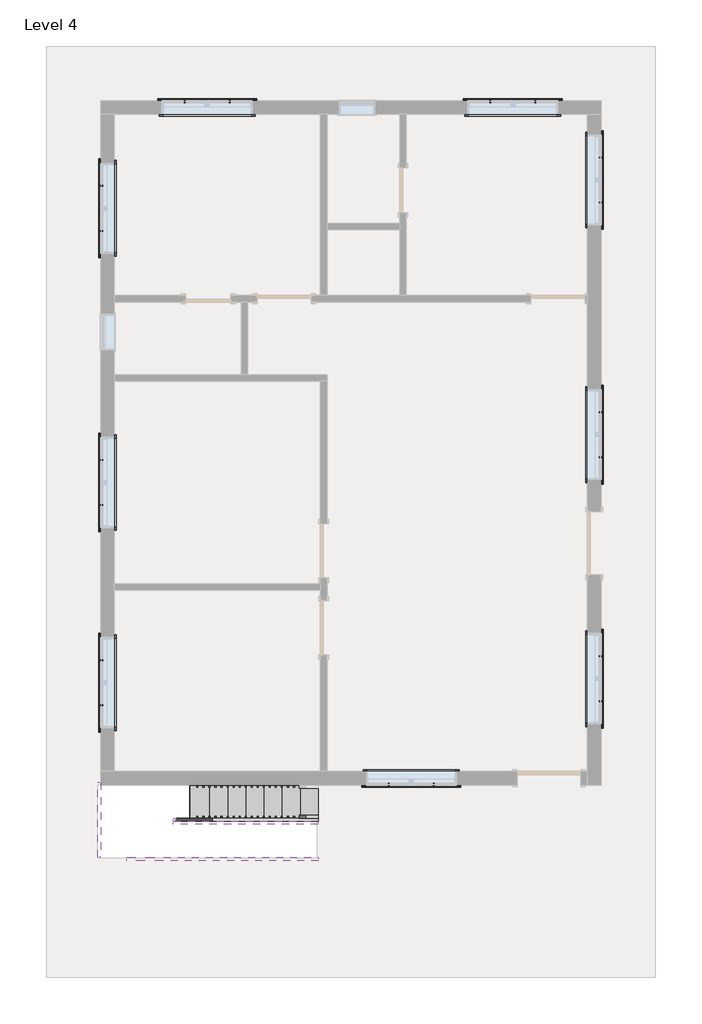
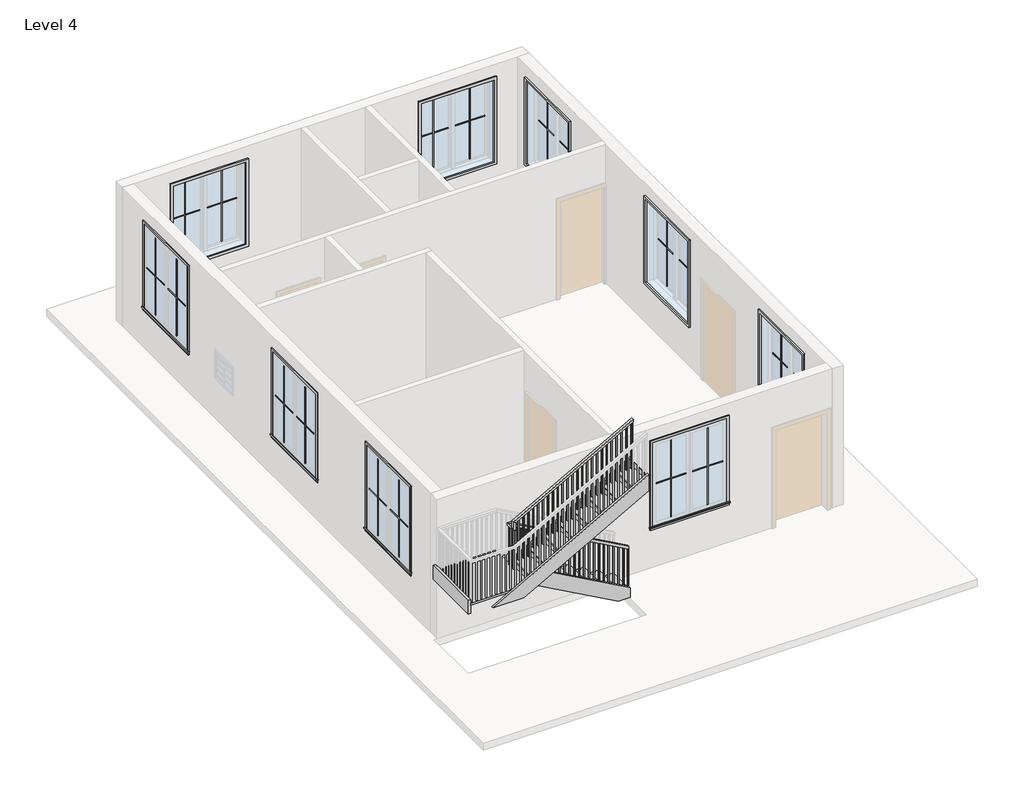
# One storey, part 3 of 3: 36 proxies, 6 members, 1 railing, 1 stair flight.
"""IFC4 building model written with IfcOpenShell, lengths in millimetres."""

from ifc_helpers import new_model, si_unit, frame, origin, place, context, project, spatial, polyline, outline, extrude, faceted_brep, transform, mapped, element, save
from components import muntin_pattern_2x2_muntin_pattern_2x2_f6a80940, muntin_pattern_2x2_muntin_pattern_2x2_09b00a1c, trim_window_exterior_flat_with_sill_698ed857, trim_window_interior_flat_picture_frame_92551a5e, stair_flight_719863f8

model = new_model("IFC4")

# Units and contexts
model_context = context("Model", 3, world=origin())
ifc_project = project(units=[si_unit("LENGTHUNIT", "METRE", prefix="MILLI")], contexts=[model_context])

# Site, building, storey
site = spatial("IfcSite", under=ifc_project)
building = spatial("IfcBuilding", under=site)
storey = spatial("IfcBuildingStorey", under=building, Name="Level 4", Elevation=6400.8)

# Proxies
placement = place(None, origin())
muntin_pattern_2x2_muntin_pattern_2x2_shape = muntin_pattern_2x2_muntin_pattern_2x2_f6a80940(model_context)
element("IfcBuildingElementProxy", 1, Name="Muntin Pattern_2x2 : Muntin Pattern_2x2", ObjectType="Muntin Pattern_2x2 : Muntin Pattern_2x2", at=placement, inside=storey, context=model_context, shape_type="MappedRepresentation", body=[
    mapped(muntin_pattern_2x2_muntin_pattern_2x2_shape, transform((-5453.9948569, -3961.7808037, 7385.05), x_axis=(0.0, 1.0, 0.0), y_axis=(-1.0, 0.0, 0.0), z_axis=(0.0, 0.0, 1.0))),
])
element("IfcBuildingElementProxy", 2, Name="Muntin Pattern_2x2 : Muntin Pattern_2x2", ObjectType="Muntin Pattern_2x2 : Muntin Pattern_2x2", at=placement, inside=storey, context=model_context, shape_type="MappedRepresentation", body=[
    mapped(muntin_pattern_2x2_muntin_pattern_2x2_shape, transform((-5453.9948569, -593.1058037, 7385.05), x_axis=(0.0, 1.0, 0.0), y_axis=(-1.0, 0.0, 0.0), z_axis=(0.0, 0.0, 1.0))),
])
element("IfcBuildingElementProxy", 3, Name="Muntin Pattern_2x2 : Muntin Pattern_2x2", ObjectType="Muntin Pattern_2x2 : Muntin Pattern_2x2", at=placement, inside=storey, context=model_context, shape_type="MappedRepresentation", body=[
    mapped(muntin_pattern_2x2_muntin_pattern_2x2_shape, transform((-5453.9948569, 4023.3441963, 7385.05), x_axis=(0.0, 1.0, 0.0), y_axis=(-1.0, 0.0, 0.0), z_axis=(0.0, 0.0, 1.0))),
])
element("IfcBuildingElementProxy", 4, Name="Muntin Pattern_2x2 : Muntin Pattern_2x2", ObjectType="Muntin Pattern_2x2 : Muntin Pattern_2x2", at=placement, inside=storey, context=model_context, shape_type="MappedRepresentation", body=[
    mapped(muntin_pattern_2x2_muntin_pattern_2x2_shape, transform((2947.0551431, 5258.4191963, 7385.05), x_axis=(0.0, -1.0, 0.0), y_axis=(1.0, 0.0, 0.0), z_axis=(0.0, 0.0, 1.0))),
])
element("IfcBuildingElementProxy", 5, Name="Muntin Pattern_2x2 : Muntin Pattern_2x2", ObjectType="Muntin Pattern_2x2 : Muntin Pattern_2x2", at=placement, inside=storey, context=model_context, shape_type="MappedRepresentation", body=[
    mapped(muntin_pattern_2x2_muntin_pattern_2x2_shape, transform((2947.0551431, 972.1691963, 7385.05), x_axis=(0.0, -1.0, 0.0), y_axis=(1.0, 0.0, 0.0), z_axis=(0.0, 0.0, 1.0))),
])
element("IfcBuildingElementProxy", 6, Name="Muntin Pattern_2x2 : Muntin Pattern_2x2", ObjectType="Muntin Pattern_2x2 : Muntin Pattern_2x2", at=placement, inside=storey, context=model_context, shape_type="MappedRepresentation", body=[
    mapped(muntin_pattern_2x2_muntin_pattern_2x2_shape, transform((2947.0551431, -3136.2808037, 7385.05), x_axis=(0.0, -1.0, 0.0), y_axis=(1.0, 0.0, 0.0), z_axis=(0.0, 0.0, 1.0))),
])
element("IfcBuildingElementProxy", 7, Name="Muntin Pattern_2x2 : Muntin Pattern_2x2", ObjectType="Muntin Pattern_2x2 : Muntin Pattern_2x2", at=placement, inside=storey, context=model_context, shape_type="MappedRepresentation", body=[
    mapped(muntin_pattern_2x2_muntin_pattern_2x2_shape, transform((141.9426431, -5296.8683037, 7385.05), x_axis=(-1.0, 0.0, 0.0), y_axis=(0.0, -1.0, 0.0), z_axis=(0.0, 0.0, 1.0))),
])
element("IfcBuildingElementProxy", 8, Name="Muntin Pattern_2x2 : Muntin Pattern_2x2", ObjectType="Muntin Pattern_2x2 : Muntin Pattern_2x2", at=placement, inside=storey, context=model_context, shape_type="MappedRepresentation", body=[
    mapped(muntin_pattern_2x2_muntin_pattern_2x2_shape, transform((1091.2676431, 6202.9816963, 7385.05), x_axis=(1.0, 0.0, 0.0), y_axis=(0.0, 1.0, 0.0), z_axis=(0.0, 0.0, 1.0))),
])
element("IfcBuildingElementProxy", 9, Name="Muntin Pattern_2x2 : Muntin Pattern_2x2", ObjectType="Muntin Pattern_2x2 : Muntin Pattern_2x2", at=placement, inside=storey, context=model_context, shape_type="MappedRepresentation", body=[
    mapped(muntin_pattern_2x2_muntin_pattern_2x2_shape, transform((-4052.2323569, 6202.9816963, 7385.05), x_axis=(1.0, 0.0, 0.0), y_axis=(0.0, 1.0, 0.0), z_axis=(0.0, 0.0, 1.0))),
])
muntin_pattern_2x2_muntin_pattern_2x2_2_shape = muntin_pattern_2x2_muntin_pattern_2x2_09b00a1c(model_context)
element("IfcBuildingElementProxy", 10, Name="Muntin Pattern_2x2 : Muntin Pattern_2x2", ObjectType="Muntin Pattern_2x2 : Muntin Pattern_2x2", at=placement, inside=storey, context=model_context, shape_type="MappedRepresentation", body=[
    mapped(muntin_pattern_2x2_muntin_pattern_2x2_2_shape, transform((-5453.9948569, -3202.9558037, 7385.05), x_axis=(0.0, -1.0, 0.0), y_axis=(1.0, 0.0, 0.0), z_axis=(0.0, 0.0, 1.0))),
])
element("IfcBuildingElementProxy", 11, Name="Muntin Pattern_2x2 : Muntin Pattern_2x2", ObjectType="Muntin Pattern_2x2 : Muntin Pattern_2x2", at=placement, inside=storey, context=model_context, shape_type="MappedRepresentation", body=[
    mapped(muntin_pattern_2x2_muntin_pattern_2x2_2_shape, transform((-5453.9948569, 165.7191963, 7385.05), x_axis=(0.0, -1.0, 0.0), y_axis=(1.0, 0.0, 0.0), z_axis=(0.0, 0.0, 1.0))),
])
element("IfcBuildingElementProxy", 12, Name="Muntin Pattern_2x2 : Muntin Pattern_2x2", ObjectType="Muntin Pattern_2x2 : Muntin Pattern_2x2", at=placement, inside=storey, context=model_context, shape_type="MappedRepresentation", body=[
    mapped(muntin_pattern_2x2_muntin_pattern_2x2_2_shape, transform((-5453.9948569, 4782.1691963, 7385.05), x_axis=(0.0, -1.0, 0.0), y_axis=(1.0, 0.0, 0.0), z_axis=(0.0, 0.0, 1.0))),
])
element("IfcBuildingElementProxy", 13, Name="Muntin Pattern_2x2 : Muntin Pattern_2x2", ObjectType="Muntin Pattern_2x2 : Muntin Pattern_2x2", at=placement, inside=storey, context=model_context, shape_type="MappedRepresentation", body=[
    mapped(muntin_pattern_2x2_muntin_pattern_2x2_2_shape, transform((2947.0551431, 4499.5941963, 7385.05), x_axis=(0.0, 1.0, 0.0), y_axis=(-1.0, 0.0, 0.0), z_axis=(0.0, 0.0, 1.0))),
])
element("IfcBuildingElementProxy", 14, Name="Muntin Pattern_2x2 : Muntin Pattern_2x2", ObjectType="Muntin Pattern_2x2 : Muntin Pattern_2x2", at=placement, inside=storey, context=model_context, shape_type="MappedRepresentation", body=[
    mapped(muntin_pattern_2x2_muntin_pattern_2x2_2_shape, transform((2947.0551431, 213.3441963, 7385.05), x_axis=(0.0, 1.0, 0.0), y_axis=(-1.0, 0.0, 0.0), z_axis=(0.0, 0.0, 1.0))),
])
element("IfcBuildingElementProxy", 15, Name="Muntin Pattern_2x2 : Muntin Pattern_2x2", ObjectType="Muntin Pattern_2x2 : Muntin Pattern_2x2", at=placement, inside=storey, context=model_context, shape_type="MappedRepresentation", body=[
    mapped(muntin_pattern_2x2_muntin_pattern_2x2_2_shape, transform((2947.0551431, -3895.1058037, 7385.05), x_axis=(0.0, 1.0, 0.0), y_axis=(-1.0, 0.0, 0.0), z_axis=(0.0, 0.0, 1.0))),
])
element("IfcBuildingElementProxy", 16, Name="Muntin Pattern_2x2 : Muntin Pattern_2x2", ObjectType="Muntin Pattern_2x2 : Muntin Pattern_2x2", at=placement, inside=storey, context=model_context, shape_type="MappedRepresentation", body=[
    mapped(muntin_pattern_2x2_muntin_pattern_2x2_2_shape, transform((-616.8823569, -5296.8683037, 7385.05), x_axis=(1.0, 0.0, 0.0), y_axis=(0.0, 1.0, 0.0), z_axis=(0.0, 0.0, 1.0))),
])
element("IfcBuildingElementProxy", 17, Name="Muntin Pattern_2x2 : Muntin Pattern_2x2", ObjectType="Muntin Pattern_2x2 : Muntin Pattern_2x2", at=placement, inside=storey, context=model_context, shape_type="MappedRepresentation", body=[
    mapped(muntin_pattern_2x2_muntin_pattern_2x2_2_shape, transform((1850.0926431, 6202.9816963, 7385.05), x_axis=(-1.0, 0.0, 0.0), y_axis=(0.0, -1.0, 0.0), z_axis=(0.0, 0.0, 1.0))),
])
element("IfcBuildingElementProxy", 18, Name="Muntin Pattern_2x2 : Muntin Pattern_2x2", ObjectType="Muntin Pattern_2x2 : Muntin Pattern_2x2", at=placement, inside=storey, context=model_context, shape_type="MappedRepresentation", body=[
    mapped(muntin_pattern_2x2_muntin_pattern_2x2_2_shape, transform((-3293.4073569, 6202.9816963, 7385.05), x_axis=(-1.0, 0.0, 0.0), y_axis=(0.0, -1.0, 0.0), z_axis=(0.0, 0.0, 1.0))),
])
trim_window_exterior_flat_with_sill_shape = trim_window_exterior_flat_with_sill_698ed857(model_context)
element("IfcBuildingElementProxy", 19, Name="Trim-Window-Exterior-Flat : with Sill", ObjectType="Trim-Window-Exterior-Flat : with Sill", at=placement, inside=storey, context=model_context, shape_type="MappedRepresentation", body=[
    mapped(trim_window_exterior_flat_with_sill_shape, transform((-5463.5198569, -3582.3683037, 9144.0), x_axis=(0.0, -1.0, 0.0), y_axis=(0.0, 0.0, 1.0), z_axis=(-1.0, 0.0, 0.0))),
])
element("IfcBuildingElementProxy", 20, Name="Trim-Window-Exterior-Flat : with Sill", ObjectType="Trim-Window-Exterior-Flat : with Sill", at=placement, inside=storey, context=model_context, shape_type="MappedRepresentation", body=[
    mapped(trim_window_exterior_flat_with_sill_shape, transform((-5463.5198569, -213.6933037, 9144.0), x_axis=(0.0, -1.0, 0.0), y_axis=(0.0, 0.0, 1.0), z_axis=(-1.0, 0.0, 0.0))),
])
element("IfcBuildingElementProxy", 21, Name="Trim-Window-Exterior-Flat : with Sill", ObjectType="Trim-Window-Exterior-Flat : with Sill", at=placement, inside=storey, context=model_context, shape_type="MappedRepresentation", body=[
    mapped(trim_window_exterior_flat_with_sill_shape, transform((-5463.5198569, 4402.7566963, 9144.0), x_axis=(0.0, -1.0, 0.0), y_axis=(0.0, 0.0, 1.0), z_axis=(-1.0, 0.0, 0.0))),
])
element("IfcBuildingElementProxy", 22, Name="Trim-Window-Exterior-Flat : with Sill", ObjectType="Trim-Window-Exterior-Flat : with Sill", at=placement, inside=storey, context=model_context, shape_type="MappedRepresentation", body=[
    mapped(trim_window_exterior_flat_with_sill_shape, transform((2956.5801431, 4879.0066963, 9144.0), x_axis=(0.0, 1.0, 0.0), y_axis=(0.0, 0.0, 1.0), z_axis=(1.0, 0.0, 0.0))),
])
element("IfcBuildingElementProxy", 23, Name="Trim-Window-Exterior-Flat : with Sill", ObjectType="Trim-Window-Exterior-Flat : with Sill", at=placement, inside=storey, context=model_context, shape_type="MappedRepresentation", body=[
    mapped(trim_window_exterior_flat_with_sill_shape, transform((2956.5801431, 592.7566963, 9144.0), x_axis=(0.0, 1.0, 0.0), y_axis=(0.0, 0.0, 1.0), z_axis=(1.0, 0.0, 0.0))),
])
element("IfcBuildingElementProxy", 24, Name="Trim-Window-Exterior-Flat : with Sill", ObjectType="Trim-Window-Exterior-Flat : with Sill", at=placement, inside=storey, context=model_context, shape_type="MappedRepresentation", body=[
    mapped(trim_window_exterior_flat_with_sill_shape, transform((2956.5801431, -3515.6933037, 9144.0), x_axis=(0.0, 1.0, 0.0), y_axis=(0.0, 0.0, 1.0), z_axis=(1.0, 0.0, 0.0))),
])
element("IfcBuildingElementProxy", 25, Name="Trim-Window-Exterior-Flat : with Sill", ObjectType="Trim-Window-Exterior-Flat : with Sill", at=placement, inside=storey, context=model_context, shape_type="MappedRepresentation", body=[
    mapped(trim_window_exterior_flat_with_sill_shape, transform((-237.4698569, -5306.3933037, 9144.0), x_axis=(1.0, 0.0, 0.0), y_axis=(0.0, 0.0, 1.0), z_axis=(0.0, -1.0, 0.0))),
])
element("IfcBuildingElementProxy", 26, Name="Trim-Window-Exterior-Flat : with Sill", ObjectType="Trim-Window-Exterior-Flat : with Sill", at=placement, inside=storey, context=model_context, shape_type="MappedRepresentation", body=[
    mapped(trim_window_exterior_flat_with_sill_shape, transform((1470.6801431, 6212.5066963, 9144.0), x_axis=(-1.0, 0.0, 0.0), y_axis=(0.0, 0.0, 1.0), z_axis=(0.0, 1.0, 0.0))),
])
element("IfcBuildingElementProxy", 27, Name="Trim-Window-Exterior-Flat : with Sill", ObjectType="Trim-Window-Exterior-Flat : with Sill", at=placement, inside=storey, context=model_context, shape_type="MappedRepresentation", body=[
    mapped(trim_window_exterior_flat_with_sill_shape, transform((-3672.8198569, 6212.5066963, 9144.0), x_axis=(-1.0, 0.0, 0.0), y_axis=(0.0, 0.0, 1.0), z_axis=(0.0, 1.0, 0.0))),
])
trim_window_interior_flat_picture_frame_shape = trim_window_interior_flat_picture_frame_92551a5e(model_context)
element("IfcBuildingElementProxy", 28, Name="Trim-Window-Interior-Flat : Picture Frame", ObjectType="Trim-Window-Interior-Flat : Picture Frame", at=placement, inside=storey, context=model_context, shape_type="MappedRepresentation", body=[
    mapped(trim_window_interior_flat_picture_frame_shape, transform((-5234.9198569, -3582.3683037, 9144.0), x_axis=(0.0, 1.0, 0.0), y_axis=(0.0, 0.0, 1.0), z_axis=(1.0, 0.0, 0.0))),
])
element("IfcBuildingElementProxy", 29, Name="Trim-Window-Interior-Flat : Picture Frame", ObjectType="Trim-Window-Interior-Flat : Picture Frame", at=placement, inside=storey, context=model_context, shape_type="MappedRepresentation", body=[
    mapped(trim_window_interior_flat_picture_frame_shape, transform((-5234.9198569, -213.6933037, 9144.0), x_axis=(0.0, 1.0, 0.0), y_axis=(0.0, 0.0, 1.0), z_axis=(1.0, 0.0, 0.0))),
])
element("IfcBuildingElementProxy", 30, Name="Trim-Window-Interior-Flat : Picture Frame", ObjectType="Trim-Window-Interior-Flat : Picture Frame", at=placement, inside=storey, context=model_context, shape_type="MappedRepresentation", body=[
    mapped(trim_window_interior_flat_picture_frame_shape, transform((-5234.9198569, 4402.7566963, 9144.0), x_axis=(0.0, 1.0, 0.0), y_axis=(0.0, 0.0, 1.0), z_axis=(1.0, 0.0, 0.0))),
])
element("IfcBuildingElementProxy", 31, Name="Trim-Window-Interior-Flat : Picture Frame", ObjectType="Trim-Window-Interior-Flat : Picture Frame", at=placement, inside=storey, context=model_context, shape_type="MappedRepresentation", body=[
    mapped(trim_window_interior_flat_picture_frame_shape, transform((2727.9801431, 4879.0066963, 9144.0), x_axis=(0.0, -1.0, 0.0), y_axis=(0.0, 0.0, 1.0), z_axis=(-1.0, 0.0, 0.0))),
])
element("IfcBuildingElementProxy", 32, Name="Trim-Window-Interior-Flat : Picture Frame", ObjectType="Trim-Window-Interior-Flat : Picture Frame", at=placement, inside=storey, context=model_context, shape_type="MappedRepresentation", body=[
    mapped(trim_window_interior_flat_picture_frame_shape, transform((2727.9801431, 592.7566963, 9144.0), x_axis=(0.0, -1.0, 0.0), y_axis=(0.0, 0.0, 1.0), z_axis=(-1.0, 0.0, 0.0))),
])
element("IfcBuildingElementProxy", 33, Name="Trim-Window-Interior-Flat : Picture Frame", ObjectType="Trim-Window-Interior-Flat : Picture Frame", at=placement, inside=storey, context=model_context, shape_type="MappedRepresentation", body=[
    mapped(trim_window_interior_flat_picture_frame_shape, transform((2727.9801431, -3515.6933037, 9144.0), x_axis=(0.0, -1.0, 0.0), y_axis=(0.0, 0.0, 1.0), z_axis=(-1.0, 0.0, 0.0))),
])
element("IfcBuildingElementProxy", 34, Name="Trim-Window-Interior-Flat : Picture Frame", ObjectType="Trim-Window-Interior-Flat : Picture Frame", at=placement, inside=storey, context=model_context, shape_type="MappedRepresentation", body=[
    mapped(trim_window_interior_flat_picture_frame_shape, transform((-237.4698569, -5077.7933037, 9144.0), x_axis=(-1.0, 0.0, 0.0), y_axis=(0.0, 0.0, 1.0), z_axis=(0.0, 1.0, 0.0))),
])
element("IfcBuildingElementProxy", 35, Name="Trim-Window-Interior-Flat : Picture Frame", ObjectType="Trim-Window-Interior-Flat : Picture Frame", at=placement, inside=storey, context=model_context, shape_type="MappedRepresentation", body=[
    mapped(trim_window_interior_flat_picture_frame_shape, transform((1470.6801431, 5983.9066963, 9144.0), x_axis=(1.0, 0.0, 0.0), y_axis=(0.0, 0.0, 1.0), z_axis=(0.0, -1.0, 0.0))),
])
element("IfcBuildingElementProxy", 36, Name="Trim-Window-Interior-Flat : Picture Frame", ObjectType="Trim-Window-Interior-Flat : Picture Frame", at=placement, inside=storey, context=model_context, shape_type="MappedRepresentation", body=[
    mapped(trim_window_interior_flat_picture_frame_shape, transform((-3672.8198569, 5983.9066963, 9144.0), x_axis=(1.0, 0.0, 0.0), y_axis=(0.0, 0.0, 1.0), z_axis=(0.0, -1.0, 0.0))),
])

# Members
element("IfcMember", 37, ObjectType="Stringer - 2\" Width", at=placement, inside=storey, context=model_context, shape_type="SweptSolid", body=[
    extrude(outline(polyline([(6400.8, -1805.9198569), (6608.3983948, -1805.9198569), (7934.8428392, -4193.5198569), (7586.1641651, -4193.5198569), (6400.8, -2059.8643597), (6400.8, -1805.9198569)])), frame((0.0, -5915.9933037, 0.0), z_axis=(0.0, 1.0, 0.0), x_axis=(0.0, 0.0, 1.0)), (0.0, 0.0, 1.0), 50.8),
])
element("IfcMember", 38, ObjectType="Stringer - 2\" Width", at=placement, inside=storey, context=model_context, shape_type="SweptSolid", body=[
    extrude(outline(polyline([(-4244.3198569, -5865.1933037), (-4193.5198569, -5865.1933037), (-4193.5198569, -5915.9933037), (-4244.3198569, -5915.9933037), (-4244.3198569, -5865.1933037)])), frame((0.0, 0.0, 7696.2), z_axis=(0.0, 0.0, 1.0), x_axis=(1.0, 0.0, 0.0)), (0.0, 0.0, 1.0), 304.8),
])
element("IfcMember", 39, ObjectType="Stringer - 2\" Width", at=placement, inside=storey, context=model_context, shape_type="SweptSolid", body=[
    extrude(outline(polyline([(8132.3983948, -4244.3198569), (7783.7197207, -4244.3198569), (9138.3863873, -1805.9198569), (9487.0650614, -1805.9198569), (8132.3983948, -4244.3198569)])), frame((0.0, -5966.7933037, 0.0), z_axis=(0.0, 1.0, 0.0), x_axis=(0.0, 0.0, 1.0)), (0.0, 0.0, 1.0), 50.8),
])
element("IfcMember", 40, ObjectType="Stringer - 2\" Width", at=placement, inside=storey, context=model_context, shape_type="SweptSolid", body=[
    extrude(outline(polyline([(6400.8, -1805.9198569), (6608.3983948, -1805.9198569), (8001.0, -4312.6027463), (8001.0, -4940.2243597), (6400.8, -2059.8643597), (6400.8, -1805.9198569)])), frame((0.0, -5306.3933037, 0.0), z_axis=(0.0, 1.0, 0.0), x_axis=(0.0, 0.0, 1.0)), (0.0, 0.0, 1.0), 50.8),
])
element("IfcMember", 41, ObjectType="Stringer - 2\" Width", at=placement, inside=storey, context=model_context, shape_type="SweptSolid", body=[
    extrude(outline(polyline([(-5514.3198569, -5255.5933037), (-5463.5198569, -5255.5933037), (-5463.5198569, -6525.5933037), (-5514.3198569, -6525.5933037), (-5514.3198569, -5255.5933037)])), frame((0.0, 0.0, 7696.2), z_axis=(0.0, 0.0, 1.0), x_axis=(1.0, 0.0, 0.0)), (0.0, 0.0, 1.0), 304.8),
])
element("IfcMember", 42, ObjectType="Stringer - 2\" Width", at=placement, inside=storey, context=model_context, shape_type="SweptSolid", body=[
    extrude(outline(polyline([(7696.2, -4401.8553541), (9138.3863873, -1805.9198569), (9487.0650614, -1805.9198569), (7696.2, -5029.4769675), (7696.2, -4401.8553541)])), frame((0.0, -6576.3933037, 0.0), z_axis=(0.0, 1.0, 0.0), x_axis=(0.0, 0.0, 1.0)), (0.0, 0.0, 1.0), 50.8),
])

# Railing
element("IfcRailing", 43, ObjectType="Handrail - Rectangular", at=placement, inside=storey, context=model_context, shape_type="SolidModel", body=[
    faceted_brep([(-1805.9198569, -5865.1933037, 7484.5333333), (-1805.9198569, -5865.1933037, 7426.420221), (-1805.9198569, -5814.3933037, 7426.420221), (-1805.9198569, -5814.3933037, 7484.5333333), (-4168.1198569, -5865.1933037, 8796.8666667), (-4218.9198569, -5865.1933037, 8766.9757765), (-4218.9198569, -5814.3933037, 8766.9757765), (-4168.1198569, -5814.3933037, 8796.8666667), (-4168.1198569, -5865.1933037, 8839.2), (-4218.9198569, -5865.1933037, 8788.4), (-4218.9198569, -5814.3933037, 8788.4), (-4168.1198569, -5814.3933037, 8839.2), (-4244.3198569, -5865.1933037, 8839.2), (-4244.3198569, -5865.1933037, 8788.4), (-4295.1198569, -5814.3933037, 8788.4), (-4295.1198569, -5814.3933037, 8839.2), (-4244.3198569, -5941.3933037, 8839.2), (-4244.3198569, -5941.3933037, 8788.4), (-4295.1198569, -5941.3933037, 8788.4), (-4295.1198569, -5941.3933037, 8839.2), (-4244.3198569, -5966.7933037, 8839.2), (-4295.1198569, -5966.7933037, 8839.2), (-4295.1198569, -6017.5933037, 8788.4), (-4244.3198569, -6017.5933037, 8788.4)], [[[0, 1, 2, 3]], [[1, 0, 4, 5]], [[2, 1, 5, 6]], [[3, 2, 6, 7]], [[0, 3, 7, 4]], [[5, 4, 8, 9]], [[6, 5, 9, 10]], [[7, 6, 10, 11]], [[4, 7, 11, 8]], [[9, 8, 12, 13]], [[10, 9, 13, 14]], [[11, 10, 14, 15]], [[8, 11, 15, 12]], [[13, 12, 16, 17]], [[14, 13, 17, 18]], [[15, 14, 18, 19]], [[12, 15, 19, 16]], [[20, 21, 22, 23]], [[17, 16, 20, 23]], [[18, 17, 23, 22]], [[19, 18, 22, 21]], [[16, 19, 21, 20]]]),
    faceted_brep([(-4244.3198569, -5966.7933037, 8839.2), (-4244.3198569, -6017.5933037, 8788.4), (-4295.1198569, -6017.5933037, 8788.4), (-4295.1198569, -5966.7933037, 8839.2), (-4244.3198569, -5966.7933037, 8950.420221), (-4295.1198569, -5966.7933037, 8980.3111111), (-4295.1198569, -6017.5933037, 8980.3111111), (-4244.3198569, -6017.5933037, 8950.420221)], [[[0, 1, 2, 3]], [[4, 5, 6, 7]], [[1, 0, 4, 7]], [[2, 1, 7, 6]], [[3, 2, 6, 5]], [[0, 3, 5, 4]]]),
    faceted_brep([(-4295.1198569, -5966.7933037, 8980.3111111), (-4244.3198569, -5966.7933037, 8950.420221), (-4244.3198569, -6017.5933037, 8950.420221), (-4295.1198569, -6017.5933037, 8980.3111111), (-1805.9198569, -5966.7933037, 10363.2), (-1805.9198569, -6017.5933037, 10363.2), (-1805.9198569, -6017.5933037, 10305.0868876), (-1805.9198569, -5966.7933037, 10305.0868876)], [[[0, 1, 2, 3]], [[4, 5, 6, 7]], [[1, 0, 4, 7]], [[2, 1, 7, 6]], [[3, 2, 6, 5]], [[0, 3, 5, 4]]]),
    extrude(outline(polyline([(10285.6841099, -1840.8448569), (9279.4666667, -1840.8448569), (9279.4666667, -1821.7948569), (10296.2674432, -1821.7948569), (10285.6841099, -1840.8448569)])), frame((0.0, -6001.7183037, 0.0), z_axis=(0.0, 1.0, 0.0), x_axis=(0.0, 0.0, 1.0)), (0.0, 0.0, 1.0), 19.05),
    extrude(outline(polyline([(10229.2396654, -1942.4448569), (9279.4666667, -1942.4448569), (9279.4666667, -1923.3948569), (10239.8229988, -1923.3948569), (10229.2396654, -1942.4448569)])), frame((0.0, -6001.7183037, 0.0), z_axis=(0.0, 1.0, 0.0), x_axis=(0.0, 0.0, 1.0)), (0.0, 0.0, 1.0), 19.05),
    extrude(outline(polyline([(10172.795221, -2044.0448569), (9279.4666667, -2044.0448569), (9279.4666667, -2024.9948569), (10183.3785543, -2024.9948569), (10172.795221, -2044.0448569)])), frame((0.0, -6001.7183037, 0.0), z_axis=(0.0, 1.0, 0.0), x_axis=(0.0, 0.0, 1.0)), (0.0, 0.0, 1.0), 19.05),
    extrude(outline(polyline([(10116.3507765, -2145.6448569), (9110.1333333, -2145.6448569), (9110.1333333, -2126.5948569), (10126.9341099, -2126.5948569), (10116.3507765, -2145.6448569)])), frame((0.0, -6001.7183037, 0.0), z_axis=(0.0, 1.0, 0.0), x_axis=(0.0, 0.0, 1.0)), (0.0, 0.0, 1.0), 19.05),
    extrude(outline(polyline([(10059.9063321, -2247.2448569), (9110.1333333, -2247.2448569), (9110.1333333, -2228.1948569), (10070.4896654, -2228.1948569), (10059.9063321, -2247.2448569)])), frame((0.0, -6001.7183037, 0.0), z_axis=(0.0, 1.0, 0.0), x_axis=(0.0, 0.0, 1.0)), (0.0, 0.0, 1.0), 19.05),
    extrude(outline(polyline([(10003.4618876, -2348.8448569), (9110.1333333, -2348.8448569), (9110.1333333, -2329.7948569), (10014.045221, -2329.7948569), (10003.4618876, -2348.8448569)])), frame((0.0, -6001.7183037, 0.0), z_axis=(0.0, 1.0, 0.0), x_axis=(0.0, 0.0, 1.0)), (0.0, 0.0, 1.0), 19.05),
    extrude(outline(polyline([(9947.0174432, -2450.4448569), (8940.8, -2450.4448569), (8940.8, -2431.3948569), (9957.6007765, -2431.3948569), (9947.0174432, -2450.4448569)])), frame((0.0, -6001.7183037, 0.0), z_axis=(0.0, 1.0, 0.0), x_axis=(0.0, 0.0, 1.0)), (0.0, 0.0, 1.0), 19.05),
    extrude(outline(polyline([(9890.5729988, -2552.0448569), (8940.8, -2552.0448569), (8940.8, -2532.9948569), (9901.1563321, -2532.9948569), (9890.5729988, -2552.0448569)])), frame((0.0, -6001.7183037, 0.0), z_axis=(0.0, 1.0, 0.0), x_axis=(0.0, 0.0, 1.0)), (0.0, 0.0, 1.0), 19.05),
    extrude(outline(polyline([(9834.1285543, -2653.6448569), (8940.8, -2653.6448569), (8940.8, -2634.5948569), (9844.7118876, -2634.5948569), (9834.1285543, -2653.6448569)])), frame((0.0, -6001.7183037, 0.0), z_axis=(0.0, 1.0, 0.0), x_axis=(0.0, 0.0, 1.0)), (0.0, 0.0, 1.0), 19.05),
    extrude(outline(polyline([(9777.6841099, -2755.2448569), (8771.4666667, -2755.2448569), (8771.4666667, -2736.1948569), (9788.2674432, -2736.1948569), (9777.6841099, -2755.2448569)])), frame((0.0, -6001.7183037, 0.0), z_axis=(0.0, 1.0, 0.0), x_axis=(0.0, 0.0, 1.0)), (0.0, 0.0, 1.0), 19.05),
    extrude(outline(polyline([(9721.2396654, -2856.8448569), (8771.4666667, -2856.8448569), (8771.4666667, -2837.7948569), (9731.8229988, -2837.7948569), (9721.2396654, -2856.8448569)])), frame((0.0, -6001.7183037, 0.0), z_axis=(0.0, 1.0, 0.0), x_axis=(0.0, 0.0, 1.0)), (0.0, 0.0, 1.0), 19.05),
    extrude(outline(polyline([(9664.795221, -2958.4448569), (8771.4666667, -2958.4448569), (8771.4666667, -2939.3948569), (9675.3785543, -2939.3948569), (9664.795221, -2958.4448569)])), frame((0.0, -6001.7183037, 0.0), z_axis=(0.0, 1.0, 0.0), x_axis=(0.0, 0.0, 1.0)), (0.0, 0.0, 1.0), 19.05),
    extrude(outline(polyline([(9608.3507765, -3060.0448569), (8602.1333333, -3060.0448569), (8602.1333333, -3040.9948569), (9618.9341099, -3040.9948569), (9608.3507765, -3060.0448569)])), frame((0.0, -6001.7183037, 0.0), z_axis=(0.0, 1.0, 0.0), x_axis=(0.0, 0.0, 1.0)), (0.0, 0.0, 1.0), 19.05),
    extrude(outline(polyline([(9551.9063321, -3161.6448569), (8602.1333333, -3161.6448569), (8602.1333333, -3142.5948569), (9562.4896654, -3142.5948569), (9551.9063321, -3161.6448569)])), frame((0.0, -6001.7183037, 0.0), z_axis=(0.0, 1.0, 0.0), x_axis=(0.0, 0.0, 1.0)), (0.0, 0.0, 1.0), 19.05),
    extrude(outline(polyline([(9495.4618876, -3263.2448569), (8602.1333333, -3263.2448569), (8602.1333333, -3244.1948569), (9506.045221, -3244.1948569), (9495.4618876, -3263.2448569)])), frame((0.0, -6001.7183037, 0.0), z_axis=(0.0, 1.0, 0.0), x_axis=(0.0, 0.0, 1.0)), (0.0, 0.0, 1.0), 19.05),
    extrude(outline(polyline([(9439.0174432, -3364.8448569), (8432.8, -3364.8448569), (8432.8, -3345.7948569), (9449.6007765, -3345.7948569), (9439.0174432, -3364.8448569)])), frame((0.0, -6001.7183037, 0.0), z_axis=(0.0, 1.0, 0.0), x_axis=(0.0, 0.0, 1.0)), (0.0, 0.0, 1.0), 19.05),
    extrude(outline(polyline([(9382.5729988, -3466.4448569), (8432.8, -3466.4448569), (8432.8, -3447.3948569), (9393.1563321, -3447.3948569), (9382.5729988, -3466.4448569)])), frame((0.0, -6001.7183037, 0.0), z_axis=(0.0, 1.0, 0.0), x_axis=(0.0, 0.0, 1.0)), (0.0, 0.0, 1.0), 19.05),
    extrude(outline(polyline([(9326.1285543, -3568.0448569), (8432.8, -3568.0448569), (8432.8, -3548.9948569), (9336.7118876, -3548.9948569), (9326.1285543, -3568.0448569)])), frame((0.0, -6001.7183037, 0.0), z_axis=(0.0, 1.0, 0.0), x_axis=(0.0, 0.0, 1.0)), (0.0, 0.0, 1.0), 19.05),
    extrude(outline(polyline([(9269.6841099, -3669.6448569), (8263.4666667, -3669.6448569), (8263.4666667, -3650.5948569), (9280.2674432, -3650.5948569), (9269.6841099, -3669.6448569)])), frame((0.0, -6001.7183037, 0.0), z_axis=(0.0, 1.0, 0.0), x_axis=(0.0, 0.0, 1.0)), (0.0, 0.0, 1.0), 19.05),
    extrude(outline(polyline([(9213.2396654, -3771.2448569), (8263.4666667, -3771.2448569), (8263.4666667, -3752.1948569), (9223.8229988, -3752.1948569), (9213.2396654, -3771.2448569)])), frame((0.0, -6001.7183037, 0.0), z_axis=(0.0, 1.0, 0.0), x_axis=(0.0, 0.0, 1.0)), (0.0, 0.0, 1.0), 19.05),
    extrude(outline(polyline([(9156.795221, -3872.8448569), (8263.4666667, -3872.8448569), (8263.4666667, -3853.7948569), (9167.3785543, -3853.7948569), (9156.795221, -3872.8448569)])), frame((0.0, -6001.7183037, 0.0), z_axis=(0.0, 1.0, 0.0), x_axis=(0.0, 0.0, 1.0)), (0.0, 0.0, 1.0), 19.05),
    extrude(outline(polyline([(9100.3507765, -3974.4448569), (8094.1333333, -3974.4448569), (8094.1333333, -3955.3948569), (9110.9341099, -3955.3948569), (9100.3507765, -3974.4448569)])), frame((0.0, -6001.7183037, 0.0), z_axis=(0.0, 1.0, 0.0), x_axis=(0.0, 0.0, 1.0)), (0.0, 0.0, 1.0), 19.05),
    extrude(outline(polyline([(9043.9063321, -4076.0448569), (8094.1333333, -4076.0448569), (8094.1333333, -4056.9948569), (9054.4896654, -4056.9948569), (9043.9063321, -4076.0448569)])), frame((0.0, -6001.7183037, 0.0), z_axis=(0.0, 1.0, 0.0), x_axis=(0.0, 0.0, 1.0)), (0.0, 0.0, 1.0), 19.05),
    extrude(outline(polyline([(8987.4618876, -4177.6448569), (8094.1333333, -4177.6448569), (8094.1333333, -4158.5948569), (8998.045221, -4158.5948569), (8987.4618876, -4177.6448569)])), frame((0.0, -6001.7183037, 0.0), z_axis=(0.0, 1.0, 0.0), x_axis=(0.0, 0.0, 1.0)), (0.0, 0.0, 1.0), 19.05),
    extrude(outline(polyline([(-4260.1948569, -5931.8683037), (-4260.1948569, -5950.9183037), (-4279.2448569, -5950.9183037), (-4279.2448569, -5931.8683037), (-4260.1948569, -5931.8683037)])), frame((0.0, 0.0, 7924.8), z_axis=(0.0, 0.0, 1.0), x_axis=(1.0, 0.0, 0.0)), (0.0, 0.0, 1.0), 863.6),
    extrude(outline(polyline([(-4234.7948569, -5849.3183037), (-4253.8448569, -5849.3183037), (-4253.8448569, -5830.2683037), (-4234.7948569, -5830.2683037), (-4234.7948569, -5849.3183037)])), frame((0.0, 0.0, 7924.8), z_axis=(0.0, 0.0, 1.0), x_axis=(1.0, 0.0, 0.0)), (0.0, 0.0, 1.0), 863.6),
    extrude(outline(polyline([(8729.9341099, -4152.2448569), (7755.4666667, -4152.2448569), (7755.4666667, -4133.1948569), (8719.3507765, -4133.1948569), (8729.9341099, -4152.2448569)])), frame((0.0, -5849.3183037, 0.0), z_axis=(0.0, 1.0, 0.0), x_axis=(0.0, 0.0, 1.0)), (0.0, 0.0, 1.0), 19.05),
    extrude(outline(polyline([(8673.4896654, -4050.6448569), (7755.4666667, -4050.6448569), (7755.4666667, -4031.5948569), (8662.9063321, -4031.5948569), (8673.4896654, -4050.6448569)])), frame((0.0, -5849.3183037, 0.0), z_axis=(0.0, 1.0, 0.0), x_axis=(0.0, 0.0, 1.0)), (0.0, 0.0, 1.0), 19.05),
    extrude(outline(polyline([(8617.045221, -3949.0448569), (7755.4666667, -3949.0448569), (7755.4666667, -3929.9948569), (8606.4618876, -3929.9948569), (8617.045221, -3949.0448569)])), frame((0.0, -5849.3183037, 0.0), z_axis=(0.0, 1.0, 0.0), x_axis=(0.0, 0.0, 1.0)), (0.0, 0.0, 1.0), 19.05),
    extrude(outline(polyline([(8560.6007765, -3847.4448569), (7586.1333333, -3847.4448569), (7586.1333333, -3828.3948569), (8550.0174432, -3828.3948569), (8560.6007765, -3847.4448569)])), frame((0.0, -5849.3183037, 0.0), z_axis=(0.0, 1.0, 0.0), x_axis=(0.0, 0.0, 1.0)), (0.0, 0.0, 1.0), 19.05),
    extrude(outline(polyline([(8504.1563321, -3745.8448569), (7586.1333333, -3745.8448569), (7586.1333333, -3726.7948569), (8493.5729988, -3726.7948569), (8504.1563321, -3745.8448569)])), frame((0.0, -5849.3183037, 0.0), z_axis=(0.0, 1.0, 0.0), x_axis=(0.0, 0.0, 1.0)), (0.0, 0.0, 1.0), 19.05),
    extrude(outline(polyline([(8447.7118876, -3644.2448569), (7586.1333333, -3644.2448569), (7586.1333333, -3625.1948569), (8437.1285543, -3625.1948569), (8447.7118876, -3644.2448569)])), frame((0.0, -5849.3183037, 0.0), z_axis=(0.0, 1.0, 0.0), x_axis=(0.0, 0.0, 1.0)), (0.0, 0.0, 1.0), 19.05),
    extrude(outline(polyline([(8391.2674432, -3542.6448569), (7416.8, -3542.6448569), (7416.8, -3523.5948569), (8380.6841099, -3523.5948569), (8391.2674432, -3542.6448569)])), frame((0.0, -5849.3183037, 0.0), z_axis=(0.0, 1.0, 0.0), x_axis=(0.0, 0.0, 1.0)), (0.0, 0.0, 1.0), 19.05),
    extrude(outline(polyline([(8334.8229988, -3441.0448569), (7416.8, -3441.0448569), (7416.8, -3421.9948569), (8324.2396654, -3421.9948569), (8334.8229988, -3441.0448569)])), frame((0.0, -5849.3183037, 0.0), z_axis=(0.0, 1.0, 0.0), x_axis=(0.0, 0.0, 1.0)), (0.0, 0.0, 1.0), 19.05),
    extrude(outline(polyline([(8278.3785543, -3339.4448569), (7416.8, -3339.4448569), (7416.8, -3320.3948569), (8267.795221, -3320.3948569), (8278.3785543, -3339.4448569)])), frame((0.0, -5849.3183037, 0.0), z_axis=(0.0, 1.0, 0.0), x_axis=(0.0, 0.0, 1.0)), (0.0, 0.0, 1.0), 19.05),
    extrude(outline(polyline([(8221.9341099, -3237.8448569), (7247.4666667, -3237.8448569), (7247.4666667, -3218.7948569), (8211.3507765, -3218.7948569), (8221.9341099, -3237.8448569)])), frame((0.0, -5849.3183037, 0.0), z_axis=(0.0, 1.0, 0.0), x_axis=(0.0, 0.0, 1.0)), (0.0, 0.0, 1.0), 19.05),
    extrude(outline(polyline([(8165.4896654, -3136.2448569), (7247.4666667, -3136.2448569), (7247.4666667, -3117.1948569), (8154.9063321, -3117.1948569), (8165.4896654, -3136.2448569)])), frame((0.0, -5849.3183037, 0.0), z_axis=(0.0, 1.0, 0.0), x_axis=(0.0, 0.0, 1.0)), (0.0, 0.0, 1.0), 19.05),
    extrude(outline(polyline([(8109.045221, -3034.6448569), (7247.4666667, -3034.6448569), (7247.4666667, -3015.5948569), (8098.4618876, -3015.5948569), (8109.045221, -3034.6448569)])), frame((0.0, -5849.3183037, 0.0), z_axis=(0.0, 1.0, 0.0), x_axis=(0.0, 0.0, 1.0)), (0.0, 0.0, 1.0), 19.05),
    extrude(outline(polyline([(8052.6007765, -2933.0448569), (7078.1333333, -2933.0448569), (7078.1333333, -2913.9948569), (8042.0174432, -2913.9948569), (8052.6007765, -2933.0448569)])), frame((0.0, -5849.3183037, 0.0), z_axis=(0.0, 1.0, 0.0), x_axis=(0.0, 0.0, 1.0)), (0.0, 0.0, 1.0), 19.05),
    extrude(outline(polyline([(7996.1563321, -2831.4448569), (7078.1333333, -2831.4448569), (7078.1333333, -2812.3948569), (7985.5729988, -2812.3948569), (7996.1563321, -2831.4448569)])), frame((0.0, -5849.3183037, 0.0), z_axis=(0.0, 1.0, 0.0), x_axis=(0.0, 0.0, 1.0)), (0.0, 0.0, 1.0), 19.05),
    extrude(outline(polyline([(7939.7118876, -2729.8448569), (7078.1333333, -2729.8448569), (7078.1333333, -2710.7948569), (7929.1285543, -2710.7948569), (7939.7118876, -2729.8448569)])), frame((0.0, -5849.3183037, 0.0), z_axis=(0.0, 1.0, 0.0), x_axis=(0.0, 0.0, 1.0)), (0.0, 0.0, 1.0), 19.05),
    extrude(outline(polyline([(7883.2674432, -2628.2448569), (6908.8, -2628.2448569), (6908.8, -2609.1948569), (7872.6841099, -2609.1948569), (7883.2674432, -2628.2448569)])), frame((0.0, -5849.3183037, 0.0), z_axis=(0.0, 1.0, 0.0), x_axis=(0.0, 0.0, 1.0)), (0.0, 0.0, 1.0), 19.05),
    extrude(outline(polyline([(7826.8229988, -2526.6448569), (6908.8, -2526.6448569), (6908.8, -2507.5948569), (7816.2396654, -2507.5948569), (7826.8229988, -2526.6448569)])), frame((0.0, -5849.3183037, 0.0), z_axis=(0.0, 1.0, 0.0), x_axis=(0.0, 0.0, 1.0)), (0.0, 0.0, 1.0), 19.05),
    extrude(outline(polyline([(7770.3785543, -2425.0448569), (6908.8, -2425.0448569), (6908.8, -2405.9948569), (7759.795221, -2405.9948569), (7770.3785543, -2425.0448569)])), frame((0.0, -5849.3183037, 0.0), z_axis=(0.0, 1.0, 0.0), x_axis=(0.0, 0.0, 1.0)), (0.0, 0.0, 1.0), 19.05),
    extrude(outline(polyline([(7713.9341099, -2323.4448569), (6739.4666667, -2323.4448569), (6739.4666667, -2304.3948569), (7703.3507765, -2304.3948569), (7713.9341099, -2323.4448569)])), frame((0.0, -5849.3183037, 0.0), z_axis=(0.0, 1.0, 0.0), x_axis=(0.0, 0.0, 1.0)), (0.0, 0.0, 1.0), 19.05),
    extrude(outline(polyline([(7657.4896654, -2221.8448569), (6739.4666667, -2221.8448569), (6739.4666667, -2202.7948569), (7646.9063321, -2202.7948569), (7657.4896654, -2221.8448569)])), frame((0.0, -5849.3183037, 0.0), z_axis=(0.0, 1.0, 0.0), x_axis=(0.0, 0.0, 1.0)), (0.0, 0.0, 1.0), 19.05),
    extrude(outline(polyline([(7601.045221, -2120.2448569), (6739.4666667, -2120.2448569), (6739.4666667, -2101.1948569), (7590.4618876, -2101.1948569), (7601.045221, -2120.2448569)])), frame((0.0, -5849.3183037, 0.0), z_axis=(0.0, 1.0, 0.0), x_axis=(0.0, 0.0, 1.0)), (0.0, 0.0, 1.0), 19.05),
    extrude(outline(polyline([(7544.6007765, -2018.6448569), (6570.1333333, -2018.6448569), (6570.1333333, -1999.5948569), (7534.0174432, -1999.5948569), (7544.6007765, -2018.6448569)])), frame((0.0, -5849.3183037, 0.0), z_axis=(0.0, 1.0, 0.0), x_axis=(0.0, 0.0, 1.0)), (0.0, 0.0, 1.0), 19.05),
    extrude(outline(polyline([(7488.1563321, -1917.0448569), (6570.1333333, -1917.0448569), (6570.1333333, -1897.9948569), (7477.5729988, -1897.9948569), (7488.1563321, -1917.0448569)])), frame((0.0, -5849.3183037, 0.0), z_axis=(0.0, 1.0, 0.0), x_axis=(0.0, 0.0, 1.0)), (0.0, 0.0, 1.0), 19.05),
    extrude(outline(polyline([(-4260.1948569, -5982.6683037), (-4260.1948569, -6001.7183037), (-4279.2448569, -6001.7183037), (-4279.2448569, -5982.6683037), (-4260.1948569, -5982.6683037)])), frame((0.0, 0.0, 7924.8), z_axis=(0.0, 0.0, 1.0), x_axis=(1.0, 0.0, 0.0)), (0.0, 0.0, 1.0), 863.6),
    extrude(outline(polyline([(-4260.1948569, -5849.3183037), (-4279.2448569, -5849.3183037), (-4279.2448569, -5830.2683037), (-4260.1948569, -5830.2683037), (-4260.1948569, -5849.3183037)])), frame((0.0, 0.0, 7924.8), z_axis=(0.0, 0.0, 1.0), x_axis=(1.0, 0.0, 0.0)), (0.0, 0.0, 1.0), 863.6),
    extrude(outline(polyline([(10294.5035543, -1824.9698569), (9279.4666667, -1824.9698569), (9279.4666667, -1805.9198569), (10305.0868876, -1805.9198569), (10294.5035543, -1824.9698569)])), frame((0.0, -6001.7183037, 0.0), z_axis=(0.0, 1.0, 0.0), x_axis=(0.0, 0.0, 1.0)), (0.0, 0.0, 1.0), 19.05),
    extrude(outline(polyline([(7437.0035543, -1824.9698569), (6570.1333333, -1824.9698569), (6570.1333333, -1805.9198569), (7426.420221, -1805.9198569), (7437.0035543, -1824.9698569)])), frame((0.0, -5849.3183037, 0.0), z_axis=(0.0, 1.0, 0.0), x_axis=(0.0, 0.0, 1.0)), (0.0, 0.0, 1.0), 19.05),
])

# Stair flight
stair_flight_shape = stair_flight_719863f8(model_context)
element("IfcStairFlight", 44, ObjectType="2\" Tread 1\" Nosing 1/4\" Riser", at=placement, inside=storey, context=model_context, shape_type="MappedRepresentation", body=[
    mapped(stair_flight_shape, transform((0.0, 0.0, 0.0), x_axis=(1.0, 0.0, 0.0), y_axis=(0.0, 1.0, 0.0), z_axis=(0.0, 0.0, 1.0))),
])

save(model, "model.ifc")

# Revit data of these elements
# Type "Muntin Pattern_2x2 : Muntin Pattern_2x2"
#   Width [instance default] = 4' - 0"
#   Thickness = 0' - 0 1/2"
#   Height [instance default] = 4' - 0"
#   Distance = 0' - 0 3/4"
#   Interior Material [instance default] = none
#   Exterior Material [instance default] = none
#   Default Elevation = 0
# Type "Trim-Window-Exterior-Flat : with Sill"
#   Trim Width = 0' - 2 1/4"
#   Trim Thickness_Picture Frame = 0' - 1 1/4"
#   Trim Thickness_with Sill = 0' - 0 3/4"
#   Sill Thickness = 0' - 1 1/4"
#   Opening Width [instance default] = 2' - 0"
#   Opening Height [instance default] = 3' - 0"
#   Default Elevation = 4' - 0"
#   Sill = yes
#   Picture Frame = no
#   Trim Material [instance default] = none
# Type "Trim-Window-Interior-Flat : Picture Frame"
#   Trim Thickness_Picture Frame = 0' - 1 1/4"
#   Trim Width = 0' - 2 1/4"
#   Trim Thickness_with Sill = 0' - 0 3/4"
#   Sill Thickness = 0' - 1 1/4"
#   Opening Width [instance default] = 2' - 0"
#   Opening Height [instance default] = 3' - 0"
#   Default Elevation = 4' - 0"
#   Sill = no
#   Picture Frame = yes
#   Trim Material [instance default] = none
# Type "Handrail - Rectangular"
#   Assembly Code = "C2010400"
#   built-in parameter 1008612 = 0.0416667 (stored number, unit not read)
#   built-in parameter 1008611 = 0.0416667 (stored number, unit not read)
#   built-in parameter 1008609 = 0.333333 (stored number, unit not read)
#   built-in parameter 1008604 = 0.166667 (stored number, unit not read)
#   built-in parameter 1008603 = 0.166667 (stored number, unit not read)
#   Railing Height = 3' - 0"
#   built-in parameter 1008630 = 2
#   built-in parameter 1008610 = 2
#   built-in parameter 1008618 = Baluster - Square : 3/4"
# Elements 1, 2, 3, 4, 5, 6, 7, 8, 9, 10, 11, 12, 13, 14, 15, 16, 17, 18 (IfcBuildingElementProxy, "Muntin Pattern_2x2 : Muntin Pattern_2x2")
#   Width = 2' - 0 5/8"
#   Height = 5' - 6 1/2"
#   Interior Material = Wood - Stained
#   Exterior Material = Clad - White
#   Phase Created = New Construction
#   Materials on its faces: "Clad - White", "Wood - Stained"
# Elements 19, 20, 21, 22, 23, 24, 25, 26, 27 (IfcBuildingElementProxy, "Trim-Window-Exterior-Flat : with Sill")
#   Opening Width = 5' - 0"
#   Opening Height = 6' - 0"
#   Trim Material = Clad - White
#   Phase Created = New Construction
#   Materials on its faces: "Clad - White"
# Elements 28, 29, 30, 31, 32, 33, 34, 35, 36 (IfcBuildingElementProxy, "Trim-Window-Interior-Flat : Picture Frame")
#   Opening Width = 5' - 0"
#   Opening Height = 6' - 0"
#   Trim Material = Wood - Stained
#   Phase Created = New Construction
#   Materials on its faces: "Wood - Stained"
# Elements 37, 38, 39, 40, 41, 42 (IfcMember, "Stringer - 2\" Width")
#   Phase Created = New Construction
# Element 43 (IfcRailing, "Handrail - Rectangular")
#   Phase Created = New Construction
# Element 44 (IfcStairFlight, "2\" Tread 1\" Nosing 1/4\" Riser")
#   Phase Created = New Construction
# Materials
#   "Clad - White": class "Wood", colour RGB 242 242 238, transparency 0, Cost = 0
#   "Wood - Stained": class "Wood", colour RGB 224 178 126, transparency 0, Cost = 0
